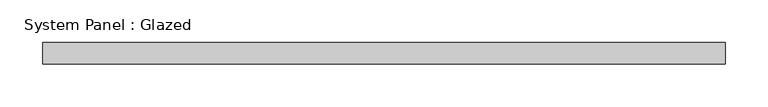
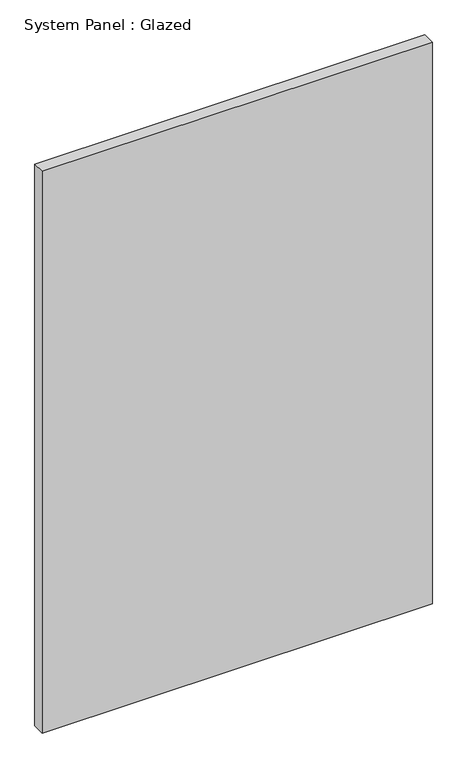
"""IFC4 building model written with IfcOpenShell, lengths in millimetres: plate geometry, System Panel : Glazed."""

from ifc_helpers import new_model, si_unit, origin, origin_with_axes, place, context, project, spatial, polyline, outline, extrude, source, transform, mapped, element, save


def system_panel_glazed_ba533b82(model_context):
    return source(origin(), model_context, "Body", "SweptSolid", [
        extrude(outline(polyline([(400.05, 19.05), (-400.05, 19.05), (-400.05, 44.45), (400.05, 44.45), (400.05, 19.05)])), origin_with_axes(), (0.0, 0.0, 1.0), 1216.8279521),
    ])


if __name__ == "__main__":
    model = new_model("IFC4")
    model_context = context("Model", 3, world=origin())
    ifc_project = project(units=[si_unit("LENGTHUNIT", "METRE", prefix="MILLI")], contexts=[model_context])
    site = spatial("IfcSite", under=ifc_project)
    building = spatial("IfcBuilding", under=site)
    placement = place(None, origin())
    system_panel_glazed_shape = system_panel_glazed_ba533b82(model_context)
    element("IfcPlate", 1, ObjectType="System Panel : Glazed", at=placement, inside=building, context=model_context, shape_type="MappedRepresentation", body=[
        mapped(system_panel_glazed_shape, transform((0.0, 0.0, 0.0), x_axis=(1.0, 0.0, 0.0), y_axis=(0.0, 1.0, 0.0), z_axis=(0.0, 0.0, 1.0))),
    ])
    save(model, "model.ifc")

# Revit data of these elements
# Type "System Panel : Glazed"
#   Construction Type Id = "GSP4R"
#   Analytic Construction = "1/8 in Pilkington single glazing"
#   Visual Light Transmittance = 0.9
#   Solar Heat Gain Coefficient = 0.86
#   Heat Transfer Coefficient (U) = 1.18115 BTU/(h·ft²·°F)
#   Define Thermal Properties by = 1
# Element 1 (IfcPlate, "System Panel : Glazed")
#   Materials on its faces: "Glass"
# Materials
#   "Glass": class "Glass", colour RGB 0 128 192, transparency 0.75, Description = "Soda Lime Glass", Cost = 0
